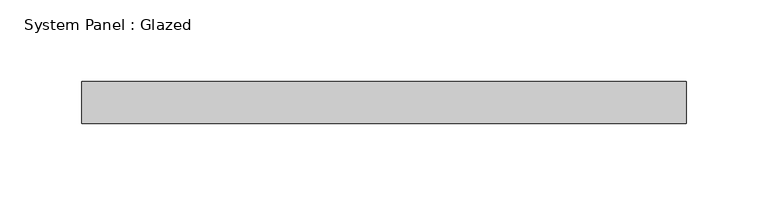
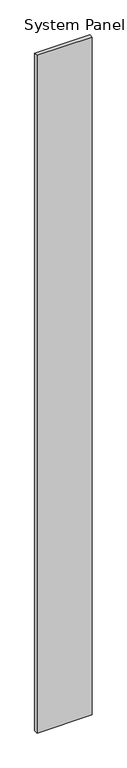
"""IFC4 building model written with IfcOpenShell, lengths in millimetres: plate geometry, System Panel : Glazed."""

from ifc_helpers import new_model, si_unit, origin, origin_with_axes, place, context, project, spatial, polyline, outline, extrude, source, transform, mapped, element, save


def system_panel_glazed_557308a9(model_context):
    return source(origin(), model_context, "Body", "SweptSolid", [
        extrude(outline(polyline([(184.15, 19.05), (-184.15, 19.05), (-184.15, 44.45), (184.15, 44.45), (184.15, 19.05)])), origin_with_axes(), (0.0, 0.0, 1.0), 4768.3171854),
    ])


if __name__ == "__main__":
    model = new_model("IFC4")
    model_context = context("Model", 3, world=origin())
    ifc_project = project(units=[si_unit("LENGTHUNIT", "METRE", prefix="MILLI")], contexts=[model_context])
    site = spatial("IfcSite", under=ifc_project)
    building = spatial("IfcBuilding", under=site)
    placement = place(None, origin())
    system_panel_glazed_shape = system_panel_glazed_557308a9(model_context)
    element("IfcPlate", 1, ObjectType="System Panel : Glazed", at=placement, inside=building, context=model_context, shape_type="MappedRepresentation", body=[
        mapped(system_panel_glazed_shape, transform((0.0, 0.0, 0.0), x_axis=(1.0, 0.0, 0.0), y_axis=(0.0, 1.0, 0.0), z_axis=(0.0, 0.0, 1.0))),
    ])
    save(model, "model.ifc")

# Revit data of these elements
# Type "System Panel : Glazed"
#   Construction Type Id = "GSP4R"
#   Analytic Construction = "1/8 in Pilkington single glazing"
#   Visual Light Transmittance = 0.9
#   Solar Heat Gain Coefficient = 0.86
#   Heat Transfer Coefficient (U) = 1.18115 BTU/(h·ft²·°F)
#   Define Thermal Properties by = 1
# Element 1 (IfcPlate, "System Panel : Glazed")
#   Materials on its faces: "Glass"
# Materials
#   "Glass": class "Glass", colour RGB 0 128 192, transparency 0.75, Description = "Soda Lime Glass", Cost = 0
